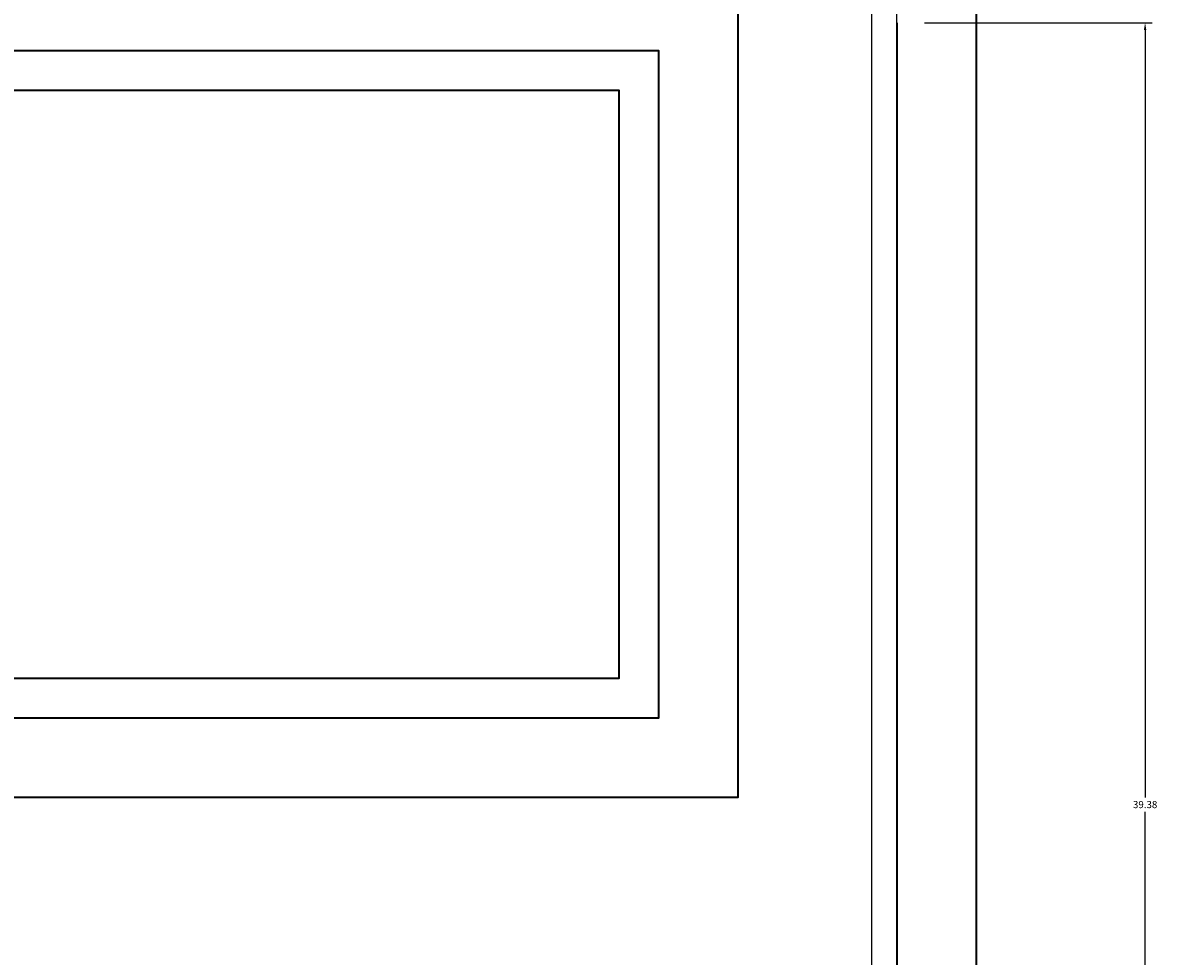
# Model space of a CAD drawing. Units: inches. Extents: x 3137 to 3299, y 1994 to 2089.
# Tile 4 of 14: x 3165 to 3194, y 2028 to 2052. Entities that reach past the tile are written whole.
import ezdxf

# ---------------------------------------------------------------- set-up
doc = ezdxf.new("R2010")
doc.units = ezdxf.units.IN
doc.header["$MEASUREMENT"] = 0
for name, color, linetype, lineweight in [('A-ANNO-DIMS', 2, 'Continuous', 18), ('A-ANNO-NPLT', 8, 'Continuous', 13), ('A-DOOR', 4, 'Continuous', 35)]:
    doc.layers.add(name, color=color, linetype=linetype, lineweight=lineweight)
doc.styles.get("Standard").update_dxf_attribs({"font": 'arial.ttf'})
doc.dimstyles.get("Standard").update_dxf_attribs({"dimtxt": 0.18, "dimasz": 0.18, "dimexe": 0.18, "dimexo": 0.0625, "dimgap": 0.09, "dimtad": 0, "dimtih": 1, "dimtoh": 1, "dimdec": 4, "dimzin": 0, "dimdsep": 46, "dimtxsty": 'Standard', "dimcen": 0.09, "dimadec": 0, "dimazin": 0, "dimtfac": 1, "dimtdec": 4, "dimtofl": 0, "dimtmove": 0, "dimatfit": 3, "dimfxl": 1, "dimtolj": 1, "dimtzin": 0, "dimarcsym": 0})

# ---------------------------------------------------------------- blocks, each defined once
blk = doc.blocks.new('*D52')
at = {"layer": 'A-ANNO-DIMS', "color": 0, "lineweight": -2, "transparency": 16777216}
for p, q in [((3188.174, 2051.649), (3193.908, 2051.649)), ((3193.728, 2051.469), (3193.728, 2032.141)), ((3193.728, 2012.449), (3193.728, 2031.777)), ((3188.18, 2012.269), (3193.908, 2012.269))]:
    blk.add_line(p, q, dxfattribs=at)
at = {"layer": 'A-ANNO-DIMS', "color": 0, "transparency": 16777216}
for points in [[(3193.698, 2051.469), (3193.758, 2051.469), (3193.728, 2051.649)], [(3193.698, 2012.449), (3193.758, 2012.449), (3193.728, 2012.269)]]:
    blk.add_solid(points, dxfattribs=at)
at = {"layer": 'Defpoints', "color": 0, "transparency": 16777216}
for p in [(3188.112, 2051.649), (3193.728, 2051.649), (3188.117, 2012.269)]:
    blk.add_point(p, dxfattribs=at)
at = {"layer": 'A-ANNO-DIMS', "color": 0, "transparency": 16777216, "insert": (3193.728, 2031.959), "char_height": 0.18, "attachment_point": 5}
blk.add_mtext('\\A1;39.38', dxfattribs=at)
blk = doc.blocks.new('*D76')
at = {"layer": 'A-ANNO-DIMS', "color": 0, "lineweight": -2, "transparency": 16777216}
for p, q in [((3186.849, 2012.332), (3186.849, 2087.304)), ((3187.478, 2012.332), (3187.478, 2087.304)), ((3187.029, 2087.124), (3187.298, 2087.124)), ((3187.478, 2087.124), (3187.658, 2087.124))]:
    blk.add_line(p, q, dxfattribs=at)
at = {"layer": 'A-ANNO-DIMS', "color": 0, "transparency": 16777216}
for points in [[(3187.029, 2087.154), (3187.029, 2087.094), (3186.849, 2087.124)], [(3187.298, 2087.154), (3187.298, 2087.094), (3187.478, 2087.124)]]:
    blk.add_solid(points, dxfattribs=at)
at = {"layer": 'Defpoints', "color": 0, "transparency": 16777216}
for p in [(3187.478, 2087.124), (3186.849, 2012.269), (3187.478, 2012.269)]:
    blk.add_point(p, dxfattribs=at)
at = {"layer": 'A-ANNO-DIMS', "color": 0, "transparency": 16777216, "insert": (3188.052, 2087.124), "char_height": 0.18, "attachment_point": 5}
blk.add_mtext('\\A1;0.628', dxfattribs=at)

msp = doc.modelspace()

# ---------------------------------------------------------------- linework, layer by layer
at = {"layer": 'A-ANNO-NPLT'}
msp.add_point((3183.4777, 2040.874), dxfattribs=at)
at = {"layer": 'A-DOOR'}
for points in [[(3141.4777, 2082.874), (3189.4777, 2082.874), (3189.4777, 1998.874), (3141.4777, 1998.874)], [(3147.4777, 2032.1375), (3147.4777, 2052.9483), (3183.4777, 2052.9483), (3183.4777, 2032.1375)], [(3149.4777, 2034.1375), (3149.4777, 2050.9483), (3181.4777, 2050.9483), (3181.4777, 2034.1375)], [(3150.4777, 2035.1375), (3150.4777, 2049.9483), (3180.4777, 2049.9483), (3180.4777, 2035.1375)]]:
    msp.add_lwpolyline(points, close=True, dxfattribs=at)
msp.add_lwpolyline([(3187.4777, 2051.6494), (3187.4777, 2012.2692)], dxfattribs=at)

# ---------------------------------------------------------------- dimensions: what is measured, and where the dimension line sits
at = {"layer": 'A-ANNO-DIMS'}
dim = msp.add_linear_dim(base=(3187.4777, 2087.124), p1=(3186.8495, 2012.2692), p2=(3187.4777, 2012.2692), dimstyle='Standard', override={"dimdec": 3, "dimlfac": 1, "dimrnd": 0, "dimzin": 0, "dimdsep": 46, "dimlunit": 2}, dxfattribs=at)
dim.commit()
dim.dimension.update_dxf_attribs({"geometry": '*D76', "text_midpoint": (3188.0516, 2087.124)})
dim = msp.add_linear_dim(base=(3193.7277, 2051.6494), p1=(3188.1173, 2012.2692), p2=(3188.1116, 2051.6494), angle=90, dimstyle='Standard', override={"dimdec": 2, "dimlfac": 1, "dimrnd": 0, "dimzin": 0, "dimdsep": 46, "dimlunit": 2}, dxfattribs=at)
dim.commit()
dim.dimension.update_dxf_attribs({"geometry": '*D52', "text_midpoint": (3193.7277, 2031.9593)})

doc.saveas('drawing.dxf')
